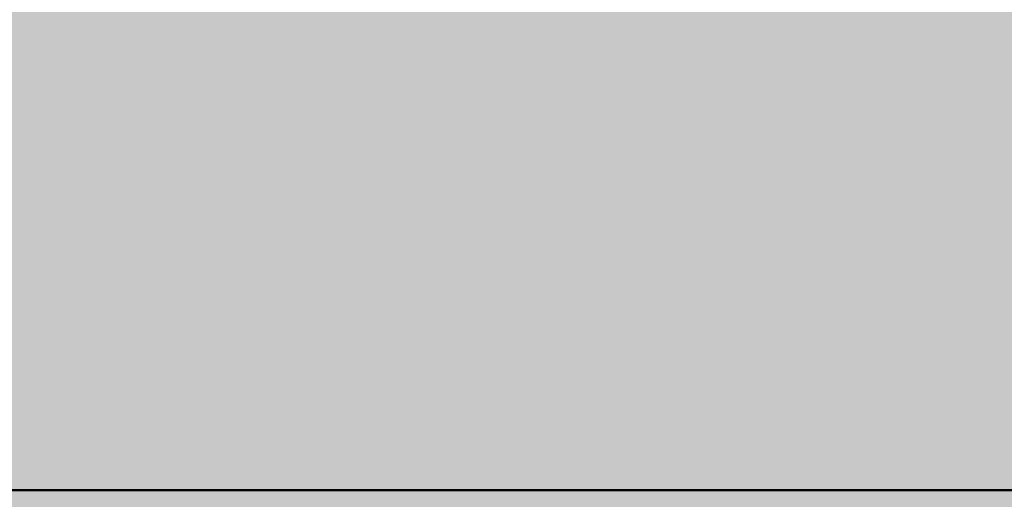
# Model space of a CAD drawing. Units: millimetres. Extents: x 0 to 2267, y 0 to 1823.
# Tile 145 of 256: x 1823.16 to 1833.61, y 1117.32 to 1122.41. Entities that reach past the tile are written whole.
import ezdxf

# ---------------------------------------------------------------- set-up
doc = ezdxf.new("R2010")
doc.units = ezdxf.units.MM
doc.header["$MEASUREMENT"] = 0
for name, color, linetype, lineweight in [('M-DIMS', 2, 'Continuous', 25), ('M-HATC', 252, 'Continuous', 18), ('M-OUTL', 7, 'Continuous', 50)]:
    doc.layers.add(name, color=color, linetype=linetype, lineweight=lineweight)
doc.styles.get("Standard").update_dxf_attribs({"font": 'arial.ttf'})
doc.dimstyles.get("Standard").update_dxf_attribs({"dimtxt": 7, "dimasz": 4, "dimexe": 0.18, "dimexo": 0.0625, "dimgap": 0.09, "dimtad": 0, "dimdec": 0, "dimzin": 0, "dimdsep": 46, "dimtxsty": 'Standard', "dimcen": 0.09, "dimadec": 0, "dimazin": 0, "dimtfac": 1, "dimtdec": 0, "dimtofl": 0, "dimtmove": 0, "dimatfit": 3, "dimfxl": 1, "dimtolj": 1, "dimtzin": 0, "dimarcsym": 0})

# ---------------------------------------------------------------- blocks, each defined once
blk = doc.blocks.new('*D1')
at = {"layer": 'Defpoints', "color": 0, "transparency": 16777216}
for p in [(1593.429, 1127.417), (1843.429, 1127.417), (1843.429, 955.628)]:
    blk.add_point(p, dxfattribs=at)
at = {"layer": 'M-DIMS', "color": 0, "lineweight": -2, "transparency": 16777216}
for p, q in [((1593.429, 1127.355), (1593.429, 955.448)), ((1843.429, 1127.355), (1843.429, 955.448)), ((1597.429, 955.628), (1710.558, 955.628)), ((1839.429, 955.628), (1726.3, 955.628))]:
    blk.add_line(p, q, dxfattribs=at)
at = {"layer": 'M-DIMS', "color": 0, "transparency": 16777216}
for points in [[(1597.429, 956.294), (1597.429, 954.961), (1593.429, 955.628)], [(1839.429, 956.294), (1839.429, 954.961), (1843.429, 955.628)]]:
    blk.add_solid(points, dxfattribs=at)
at = {"layer": 'M-DIMS', "color": 0, "transparency": 16777216, "insert": (1718.429, 955.628), "char_height": 7, "attachment_point": 5}
blk.add_mtext('\\A1;250', dxfattribs=at)

msp = doc.modelspace()

# ---------------------------------------------------------------- hatches: boundary and pattern name
at = {"layer": 'M-HATC'}
h = msp.add_hatch(color=256, dxfattribs=at)
h.dxf.hatch_style = 1
h.paths.add_polyline_path([(2065.771, 1618.062, 0.236068), (2055.771, 1638.062), (1381.087, 1638.062, 0.236068), (1371.087, 1618.062), (1371.087, 1603.062), (2055.771, 1603.062), (2065.771, 1603.062)])
h.paths.add_polyline_path([(2062.772, 1550.296), (2062.772, 1560.296), (1374.086, 1560.296), (1374.086, 1550.296), (1374.086, 1540.296), (1384.086, 1540.296), (1389.086, 1540.296), (2062.772, 1540.296)])
h.paths.add_polyline_path([(1930.929, 1282.766), (1505.929, 1282.766), (1587.628, 1235.597, 0.131652), (1600.128, 1232.247), (1836.73, 1232.247, 0.131652), (1849.23, 1235.597)])
h.paths.add_polyline_path([(1930.929, 1117.417), (1905.929, 1117.417), (1505.929, 1117.417), (1505.929, 1077.417), (1930.929, 1077.417)])
h = msp.add_hatch(color=256, dxfattribs=at)
h.dxf.hatch_style = 1
h.paths.add_polyline_path([(2055.771, 1603.062), (1381.087, 1603.062), (1381.087, 1598.062), (2055.771, 1598.062)])
h.paths.add_polyline_path([(2055.771, 1598.062), (1381.087, 1598.062), (1381.087, 1593.062), (2055.771, 1593.062)])
h.paths.add_polyline_path([(2051.307, 1536.761), (1385.55, 1536.761), (1385.55, 1526.761), (1387.55, 1526.761), (1388.537, 1525.053), (1385.332, 1521.233), (1385.332, 1521.223), (2050.254, 1522.749), (2048.321, 1525.053), (2049.307, 1526.761), (2051.307, 1526.761)])
edge = h.paths.add_edge_path()
edge.add_arc((1847.535, 1379.149), 135, 222.60306, 222.89085, ccw=False)
edge.add_line((1748.166, 1287.766), (1683.092, 1287.766))
edge.add_arc((1583.724, 1379.149), 135, 317.10915, 317.39694, ccw=False)
edge.add_arc((1678.969, 1290.671), 5, 222.8909, 317.1091, ccw=False)
edge.add_arc((1774.213, 1379.149), 135, 222.60306, 222.89085, ccw=False)
edge.add_line((1674.845, 1287.766), (1609.771, 1287.766))
edge.add_arc((1510.403, 1379.149), 135, 317.10915, 317.39694, ccw=False)
edge.add_arc((1605.647, 1290.671), 5, 222.8909, 317.1091, ccw=False)
edge.add_arc((1700.892, 1379.149), 135, 222.60306, 222.89085, ccw=False)
edge.add_line((1601.524, 1287.766), (1536.45, 1287.766))
edge.add_arc((1437.081, 1379.149), 135, 317.10915, 317.39694, ccw=False)
edge.add_arc((1532.326, 1290.671), 5, 222.8909, 317.1091, ccw=False)
edge.add_arc((1627.571, 1379.149), 135, 222.60306, 222.89085, ccw=False)
edge.add_line((1528.203, 1287.766), (1505.929, 1287.766))
edge.add_spline(control_points=[(1505.929, 1287.766), (1504.262, 1287.766), (1504.262, 1282.766), (1505.929, 1282.766)], knot_values=[0, 0, 0, 0, 5, 5, 5, 5], degree=3, periodic=0)
edge.add_line((1505.929, 1282.766), (1930.929, 1282.766))
edge.add_spline(control_points=[(1930.929, 1282.766), (1932.596, 1282.766), (1932.596, 1287.766), (1930.929, 1287.766)], knot_values=[0, 0, 0, 0, 5, 5, 5, 5], degree=3, periodic=0)
edge.add_line((1930.929, 1287.766), (1903.056, 1287.766))
edge.add_arc((1803.688, 1379.149), 135, 317.10915, 317.39694, ccw=False)
edge.add_arc((1898.932, 1290.671), 5, 222.8909, 317.1091, ccw=False)
edge.add_arc((1994.177, 1379.149), 135, 222.60306, 222.89085, ccw=False)
edge.add_line((1894.809, 1287.766), (1829.735, 1287.766))
edge.add_arc((1730.366, 1379.149), 135, 317.10915, 317.39694, ccw=False)
edge.add_arc((1825.611, 1290.671), 5, 222.8909, 317.1091, ccw=False)
edge.add_arc((1920.856, 1379.149), 135, 222.60306, 222.89085, ccw=False)
edge.add_line((1821.487, 1287.766), (1756.413, 1287.766))
edge.add_arc((1657.045, 1379.149), 135, 317.10915, 317.39694, ccw=False)
edge.add_arc((1752.29, 1290.671), 5, 222.8909, 317.1091, ccw=False)
edge = h.paths.add_edge_path()
edge.add_spline(control_points=[(1843.429, 1227.247), (1845.096, 1227.247), (1845.096, 1232.247), (1843.429, 1232.247)], knot_values=[0, 0, 0, 0, 5, 5, 5, 5], degree=3, periodic=0)
edge.add_line((1843.429, 1232.247), (1593.429, 1232.247))
edge.add_spline(control_points=[(1593.429, 1232.247), (1591.762, 1232.247), (1591.762, 1227.247), (1593.429, 1227.247)], knot_values=[0, 0, 0, 0, 5, 5, 5, 5], degree=3, periodic=0)
edge.add_line((1593.429, 1227.247), (1843.429, 1227.247))
h.paths.add_polyline_path([(1905.929, 1127.417), (1530.929, 1127.417, 0.414214), (1520.929, 1117.417), (1530.929, 1117.417), (1915.929, 1117.417, 0.414214)])
edge = h.paths.add_edge_path()
edge.add_arc((1397.086, 1498.408), 12.73, 90.7821, 190.8787, ccw=False)
edge.add_line((1396.912, 1511.136), (1428.01, 1511.349))
edge.add_line((1428.01, 1511.349), (1433.01, 1511.349))
edge.add_line((1433.01, 1511.349), (1434.439, 1511.349))
edge.add_arc((1419.474, 1498.08), 20, 41.561, 74.0821)
edge.add_line((1424.959, 1517.314), (1399.935, 1517.256))
edge.add_spline(control_points=[(1399.931, 1517.256), (1399.884, 1517.213), (1399.833, 1517.169), (1399.777, 1517.124)], knot_values=[11.567499, 11.567499, 11.567499, 11.567499, 11.814249, 11.814249, 11.814249, 11.814249], degree=3, periodic=0)
edge.add_spline(control_points=[(1399.633, 1517.01), (1399.583, 1516.972), (1399.531, 1516.934), (1399.476, 1516.895)], knot_values=[11.167718, 11.167718, 11.167718, 11.167718, 11.365188, 11.365188, 11.365188, 11.365188], degree=3, periodic=0)
edge.add_spline(control_points=[(1399.34, 1516.8), (1399.151, 1516.672), (1398.938, 1516.538), (1398.704, 1516.399)], knot_values=[10.376405, 10.376405, 10.376405, 10.376405, 11.00994, 11.00994, 11.00994, 11.00994], degree=3, periodic=0)
edge.add_spline(control_points=[(1398.657, 1516.372), (1398.579, 1516.326), (1398.498, 1516.28), (1398.415, 1516.233)], knot_values=[10.125175, 10.125175, 10.125175, 10.125175, 10.334406, 10.334406, 10.334406, 10.334406], degree=3, periodic=0)
edge.add_spline(control_points=[(1398.264, 1516.149), (1398.196, 1516.111), (1398.126, 1516.073), (1398.055, 1516.035)], knot_values=[9.832246, 9.832246, 9.832246, 9.832246, 9.999658, 9.999658, 9.999658, 9.999658], degree=3, periodic=0)
edge.add_spline(control_points=[(1397.999, 1516.005), (1397.731, 1515.862), (1397.446, 1515.717), (1397.147, 1515.571)], knot_values=[9.161808, 9.161808, 9.161808, 9.161808, 9.787769, 9.787769, 9.787769, 9.787769], degree=3, periodic=0)
edge.add_spline(control_points=[(1397.147, 1515.571), (1396.842, 1515.423), (1396.522, 1515.274), (1396.191, 1515.126)], knot_values=[8.524455, 8.524455, 8.524455, 8.524455, 9.161808, 9.161808, 9.161808, 9.161808], degree=3, periodic=0)
edge.add_spline(control_points=[(1396.078, 1515.076), (1395.985, 1515.035), (1395.892, 1514.994), (1395.798, 1514.953)], knot_values=[8.275193, 8.275193, 8.275193, 8.275193, 8.451726, 8.451726, 8.451726, 8.451726], degree=3, periodic=0)
edge.add_spline(control_points=[(1395.602, 1514.869), (1395.5, 1514.826), (1395.397, 1514.782), (1395.293, 1514.739)], knot_values=[7.962917, 7.962917, 7.962917, 7.962917, 8.152764, 8.152764, 8.152764, 8.152764], degree=3, periodic=0)
edge.add_spline(control_points=[(1395.212, 1514.706), (1394.828, 1514.547), (1394.435, 1514.393), (1394.036, 1514.244)], knot_values=[7.21254, 7.21254, 7.21254, 7.21254, 7.913148, 7.913148, 7.913148, 7.913148], degree=3, periodic=0)
edge.add_spline(control_points=[(1394.036, 1514.244), (1393.708, 1514.121), (1393.375, 1514.003), (1393.043, 1513.889)], knot_values=[6.633733, 6.633733, 6.633733, 6.633733, 7.21254, 7.21254, 7.21254, 7.21254], degree=3, periodic=0)
edge.add_spline(control_points=[(1392.821, 1513.815), (1392.72, 1513.781), (1392.618, 1513.748), (1392.517, 1513.715)], knot_values=[6.328796, 6.328796, 6.328796, 6.328796, 6.505493, 6.505493, 6.505493, 6.505493], degree=3, periodic=0)
edge.add_spline(control_points=[(1392.517, 1513.715), (1392.319, 1513.652), (1392.121, 1513.59), (1391.924, 1513.531)], knot_values=[5.984605, 5.984605, 5.984605, 5.984605, 6.328796, 6.328796, 6.328796, 6.328796], degree=3, periodic=0)
edge.add_spline(control_points=[(1391.792, 1513.491), (1391.312, 1513.35), (1390.838, 1513.224), (1390.378, 1513.117)], knot_values=[5.066697, 5.066697, 5.066697, 5.066697, 5.907055, 5.907055, 5.907055, 5.907055], degree=3, periodic=0)
edge.add_spline(control_points=[(1390.378, 1513.117), (1390.18, 1513.071), (1389.984, 1513.028), (1389.791, 1512.99)], knot_values=[4.70367, 4.70367, 4.70367, 4.70367, 5.066695, 5.066695, 5.066695, 5.066695], degree=3, periodic=0)
edge.add_spline(control_points=[(1389.422, 1512.92), (1389.246, 1512.889), (1389.073, 1512.862), (1388.904, 1512.838)], knot_values=[4.130571, 4.130571, 4.130571, 4.130571, 4.469816, 4.469816, 4.469816, 4.469816], degree=3, periodic=0)
edge.add_spline(control_points=[(1388.904, 1512.838), (1388.591, 1512.795), (1388.291, 1512.764), (1388.007, 1512.749)], knot_values=[3.504031, 3.504031, 3.504031, 3.504031, 4.130571, 4.130571, 4.130571, 4.130571], degree=3, periodic=0)
edge.add_spline(control_points=[(1387.936, 1512.746), (1387.854, 1512.742), (1387.773, 1512.74), (1387.694, 1512.739)], knot_values=[3.268866, 3.268866, 3.268866, 3.268866, 3.451164, 3.451164, 3.451164, 3.451164], degree=3, periodic=0)
edge.add_spline(control_points=[(1387.335, 1512.744), (1387.208, 1512.75), (1387.085, 1512.76), (1386.967, 1512.774)], knot_values=[2.670686, 2.670686, 2.670686, 2.670686, 2.984, 2.984, 2.984, 2.984], degree=3, periodic=0)
edge.add_spline(control_points=[(1386.833, 1512.792), (1386.821, 1512.794), (1386.809, 1512.796), (1386.797, 1512.798)], knot_values=[2.516981, 2.516981, 2.516981, 2.516981, 2.549528, 2.549528, 2.549528, 2.549528], degree=3, periodic=0)
edge.add_spline(control_points=[(1386.453, 1512.873), (1386.426, 1512.881), (1386.399, 1512.889), (1386.373, 1512.897)], knot_values=[2.095869, 2.095869, 2.095869, 2.095869, 2.17941, 2.17941, 2.17941, 2.17941], degree=3, periodic=0)
edge.add_spline(control_points=[(1386.069, 1513.019), (1386.063, 1513.022), (1386.058, 1513.025), (1386.052, 1513.028)], knot_values=[1.72453, 1.72453, 1.72453, 1.72453, 1.745933, 1.745933, 1.745933, 1.745933], degree=3, periodic=0)
edge.add_arc((1399.474, 1498.08), 20, 131.8243, 180)
edge.add_arc((1630.334, 1505.548), 250.971, 181.70518, 236.42798)
edge.add_arc((1605.34, 1483.304), 218.782, 238.66083, 243.34961)
edge.add_arc((1647.091, 1510.359), 262.899, 183.12984, 237.85344, ccw=False)
h.paths.add_polyline_path([(1406.537, 1391.964, 0.149382), (1491.551, 1296.442, -0.129517)], flags=17)
edge = h.paths.add_edge_path()
edge.add_arc((2037.384, 1498.08), 20, 0, 48.2659)
edge.add_spline(control_points=[(2050.697, 1513.005), (2050.651, 1512.985), (2050.603, 1512.966), (2050.554, 1512.948)], knot_values=[1.835652, 1.835652, 1.835652, 1.835652, 2.000781, 2.000781, 2.000781, 2.000781], degree=3, periodic=0)
edge.add_spline(control_points=[(2050.462, 1512.917), (2050.479, 1512.922), (2050.496, 1512.928), (2050.513, 1512.934)], knot_values=[2.045477, 2.045477, 2.045477, 2.045477, 2.101389, 2.101389, 2.101389, 2.101389], degree=3, periodic=0)
edge.add_spline(control_points=[(2050.129, 1512.834), (2050.198, 1512.847), (2050.266, 1512.862), (2050.331, 1512.879)], knot_values=[2.237629, 2.237629, 2.237629, 2.237629, 2.435841, 2.435841, 2.435841, 2.435841], degree=3, periodic=0)
edge.add_spline(control_points=[(2050.095, 1512.828), (2050.106, 1512.83), (2050.118, 1512.832), (2050.129, 1512.834)], knot_values=[2.435841, 2.435841, 2.435841, 2.435841, 2.468321, 2.468321, 2.468321, 2.468321], degree=3, periodic=0)
edge.add_spline(control_points=[(2049.784, 1512.785), (2049.855, 1512.792), (2049.924, 1512.801), (2049.992, 1512.811)], knot_values=[2.563852, 2.563852, 2.563852, 2.563852, 2.748541, 2.748541, 2.748541, 2.748541], degree=3, periodic=0)
edge.add_spline(control_points=[(2049.405, 1512.762), (2049.536, 1512.765), (2049.663, 1512.773), (2049.784, 1512.785)], knot_values=[2.748541, 2.748541, 2.748541, 2.748541, 3.064882, 3.064882, 3.064882, 3.064882], degree=3, periodic=0)
edge.add_spline(control_points=[(2049.17, 1512.76), (2049.234, 1512.759), (2049.297, 1512.759), (2049.358, 1512.761)], knot_values=[3.102309, 3.102309, 3.102309, 3.102309, 3.2503, 3.2503, 3.2503, 3.2503], degree=3, periodic=0)
edge.add_spline(control_points=[(2048.857, 1512.769), (2048.964, 1512.764), (2049.068, 1512.761), (2049.17, 1512.76)], knot_values=[3.2503, 3.2503, 3.2503, 3.2503, 3.486069, 3.486069, 3.486069, 3.486069], degree=3, periodic=0)
edge.add_spline(control_points=[(2048.692, 1512.779), (2048.373, 1512.801), (2048.035, 1512.841), (2047.682, 1512.897)], knot_values=[3.606429, 3.606429, 3.606429, 3.606429, 4.2989, 4.2989, 4.2989, 4.2989], degree=3, periodic=0)
edge.add_spline(control_points=[(2047.682, 1512.897), (2047.546, 1512.919), (2047.408, 1512.942), (2047.268, 1512.969)], knot_values=[4.2989, 4.2989, 4.2989, 4.2989, 4.565769, 4.565769, 4.565769, 4.565769], degree=3, periodic=0)
edge.add_spline(control_points=[(2047.268, 1512.969), (2047.145, 1512.991), (2047.021, 1513.016), (2046.895, 1513.042)], knot_values=[4.565769, 4.565769, 4.565769, 4.565769, 4.799971, 4.799971, 4.799971, 4.799971], degree=3, periodic=0)
edge.add_spline(control_points=[(2046.895, 1513.042), (2046.529, 1513.119), (2046.151, 1513.209), (2045.768, 1513.311)], knot_values=[4.799971, 4.799971, 4.799971, 4.799971, 5.483718, 5.483718, 5.483718, 5.483718], degree=3, periodic=0)
edge.add_spline(control_points=[(2045.768, 1513.311), (2045.372, 1513.415), (2044.97, 1513.532), (2044.566, 1513.659)], knot_values=[5.483718, 5.483718, 5.483718, 5.483718, 6.187866, 6.187866, 6.187866, 6.187866], degree=3, periodic=0)
edge.add_spline(control_points=[(2044.566, 1513.659), (2044.415, 1513.706), (2044.263, 1513.755), (2044.112, 1513.805)], knot_values=[6.187866, 6.187866, 6.187866, 6.187866, 6.451551, 6.451551, 6.451551, 6.451551], degree=3, periodic=0)
edge.add_spline(control_points=[(2044.112, 1513.805), (2043.997, 1513.843), (2043.882, 1513.881), (2043.767, 1513.92)], knot_values=[6.451551, 6.451551, 6.451551, 6.451551, 6.651434, 6.651434, 6.651434, 6.651434], degree=3, periodic=0)
edge.add_spline(control_points=[(2043.767, 1513.92), (2043.372, 1514.055), (2042.977, 1514.198), (2042.589, 1514.346)], knot_values=[6.651434, 6.651434, 6.651434, 6.651434, 7.338879, 7.338879, 7.338879, 7.338879], degree=3, periodic=0)
edge.add_spline(control_points=[(2042.589, 1514.346), (2042.164, 1514.507), (2041.746, 1514.675), (2041.341, 1514.846)], knot_values=[7.338879, 7.338879, 7.338879, 7.338879, 8.089209, 8.089209, 8.089209, 8.089209], degree=3, periodic=0)
edge.add_spline(control_points=[(2041.341, 1514.846), (2041.103, 1514.946), (2040.869, 1515.048), (2040.64, 1515.15)], knot_values=[8.089209, 8.089209, 8.089209, 8.089209, 8.529587, 8.529587, 8.529587, 8.529587], degree=3, periodic=0)
edge.add_spline(control_points=[(2040.51, 1515.209), (2040.082, 1515.402), (2039.675, 1515.597), (2039.295, 1515.789)], knot_values=[8.613818, 8.613818, 8.613818, 8.613818, 9.44571, 9.44571, 9.44571, 9.44571], degree=3, periodic=0)
edge.add_spline(control_points=[(2039.295, 1515.789), (2039.062, 1515.907), (2038.839, 1516.025), (2038.629, 1516.14)], knot_values=[9.44571, 9.44571, 9.44571, 9.44571, 9.956404, 9.956404, 9.956404, 9.956404], degree=3, periodic=0)
edge.add_spline(control_points=[(2038.629, 1516.14), (2038.519, 1516.2), (2038.412, 1516.26), (2038.309, 1516.319)], knot_values=[9.956404, 9.956404, 9.956404, 9.956404, 10.223542, 10.223542, 10.223542, 10.223542], degree=3, periodic=0)
edge.add_spline(control_points=[(2038.309, 1516.319), (2038.214, 1516.374), (2038.122, 1516.428), (2038.033, 1516.481)], knot_values=[10.223542, 10.223542, 10.223542, 10.223542, 10.47051, 10.47051, 10.47051, 10.47051], degree=3, periodic=0)
edge.add_spline(control_points=[(2038.033, 1516.481), (2037.786, 1516.63), (2037.564, 1516.773), (2037.372, 1516.909)], knot_values=[10.47051, 10.47051, 10.47051, 10.47051, 11.15767, 11.15767, 11.15767, 11.15767], degree=3, periodic=0)
edge.add_spline(control_points=[(2037.372, 1516.909), (2037.279, 1516.975), (2037.193, 1517.04), (2037.114, 1517.102)], knot_values=[11.15767, 11.15767, 11.15767, 11.15767, 11.49227, 11.49227, 11.49227, 11.49227], degree=3, periodic=0)
edge.add_spline(control_points=[(2036.856, 1517.326), (2036.915, 1517.269), (2036.981, 1517.21), (2037.056, 1517.149)], knot_values=[11.577341, 11.577341, 11.577341, 11.577341, 11.91035, 11.91035, 11.91035, 11.91035], degree=3, periodic=0)
edge.add_spline(control_points=[(2036.807, 1517.375), (2036.823, 1517.359), (2036.839, 1517.342), (2036.856, 1517.326)], knot_values=[11.91035, 11.91035, 11.91035, 11.91035, 12.007402, 12.007402, 12.007402, 12.007402], degree=3, periodic=0)
edge.add_spline(control_points=[(2036.702, 1517.494), (2036.71, 1517.483), (2036.72, 1517.472), (2036.729, 1517.461)], knot_values=[12.184155, 12.184155, 12.184155, 12.184155, 12.255409, 12.255409, 12.255409, 12.255409], degree=3, periodic=0)
edge.add_spline(control_points=[(2036.616, 1517.621), (2036.62, 1517.613), (2036.624, 1517.606), (2036.629, 1517.598)], knot_values=[12.487913, 12.487913, 12.487913, 12.487913, 12.541035, 12.541035, 12.541035, 12.541035], degree=3, periodic=0)
edge.add_spline(control_points=[(2036.563, 1517.786), (2036.564, 1517.779), (2036.564, 1517.773), (2036.565, 1517.766)], knot_values=[12.911761, 12.911761, 12.911761, 12.911761, 12.968286, 12.968286, 12.968286, 12.968286], degree=3, periodic=0)
edge.add_spline(control_points=[(2036.617, 1517.93), (2036.612, 1517.926), (2036.609, 1517.921), (2036.605, 1517.916)], knot_values=[13.382527, 13.382527, 13.382527, 13.382527, 13.433791, 13.433791, 13.433791, 13.433791], degree=3, periodic=0)
edge.add_spline(control_points=[(2036.749, 1518.017), (2036.736, 1518.012), (2036.724, 1518.006), (2036.712, 1518)], knot_values=[13.726299, 13.726299, 13.726299, 13.726299, 13.809928, 13.809928, 13.809928, 13.809928], degree=3, periodic=0)
edge.add_spline(control_points=[(2036.86, 1518.053), (2036.839, 1518.047), (2036.818, 1518.042), (2036.799, 1518.035)], knot_values=[13.910887, 13.910887, 13.910887, 13.910887, 14.02153, 14.02153, 14.02153, 14.02153], degree=3, periodic=0)
edge.add_line((2036.964, 1518.08), (2032.384, 1518.08))
edge.add_line((2032.384, 1518.08), (2027.384, 1518.08))
edge.add_line((2027.384, 1518.08), (2022.384, 1518.08))
edge.add_line((2022.384, 1518.08), (2017.384, 1518.08))
edge.add_arc((2017.384, 1498.08), 20, 90, 138.439)
edge.add_line((2002.419, 1511.349), (2003.848, 1511.349))
edge.add_line((2003.848, 1511.349), (2008.848, 1511.349))
edge.add_line((2008.848, 1511.349), (2039.772, 1511.138))
edge.add_arc((2039.772, 1498.408), 12.73, -10.8787, 90, ccw=False)
edge.add_arc((1789.767, 1510.359), 262.899, 302.14656, 356.87016, ccw=False)
edge.add_arc((1831.518, 1483.304), 218.782, 296.65039, 301.33917)
edge.add_arc((1806.524, 1505.548), 250.971, 303.57202, 358.29482)
h.paths.add_polyline_path([(2030.321, 1391.964, -0.129517), (1945.307, 1296.442, 0.149382)], flags=17)
edge = h.paths.add_edge_path()
edge.add_spline(control_points=[(2037.246, 1518.082), (2037.29, 1518.081), (2037.336, 1518.08), (2037.384, 1518.08)], knot_values=[0.000012, 0.000012, 0.000012, 0.000012, 0.144754, 0.144754, 0.144754, 0.144754], degree=3, periodic=0)
edge.add_line((2037.336, 1518.08), (2037.01, 1518.08))
edge.add_spline(control_points=[(2037.01, 1518.08), (2036.982, 1518.077), (2036.956, 1518.073), (2036.931, 1518.068)], knot_values=[14.13465, 14.13465, 14.13465, 14.13465, 14.247197, 14.247197, 14.247197, 14.247197], degree=3, periodic=0)
edge.add_spline(control_points=[(2036.931, 1518.068), (2036.928, 1518.067), (2036.924, 1518.067), (2036.921, 1518.066)], knot_values=[14.118315, 14.118315, 14.118315, 14.118315, 14.13465, 14.13465, 14.13465, 14.13465], degree=3, periodic=0)
edge.add_spline(control_points=[(2036.921, 1518.066), (2036.912, 1518.064), (2036.903, 1518.063), (2036.895, 1518.061)], knot_values=[14.078086, 14.078086, 14.078086, 14.078086, 14.118315, 14.118315, 14.118315, 14.118315], degree=3, periodic=0)
edge.add_spline(control_points=[(2036.895, 1518.061), (2036.883, 1518.058), (2036.872, 1518.056), (2036.86, 1518.053)], knot_values=[14.02153, 14.02153, 14.02153, 14.02153, 14.078086, 14.078086, 14.078086, 14.078086], degree=3, periodic=0)
edge.add_spline(control_points=[(2036.86, 1518.053), (2036.839, 1518.047), (2036.818, 1518.042), (2036.799, 1518.035)], knot_values=[13.910887, 13.910887, 13.910887, 13.910887, 14.02153, 14.02153, 14.02153, 14.02153], degree=3, periodic=0)
edge.add_spline(control_points=[(2036.799, 1518.035), (2036.798, 1518.035), (2036.797, 1518.035), (2036.797, 1518.035)], knot_values=[13.906906, 13.906906, 13.906906, 13.906906, 13.910887, 13.910887, 13.910887, 13.910887], degree=3, periodic=0)
edge.add_spline(control_points=[(2036.797, 1518.035), (2036.788, 1518.032), (2036.78, 1518.029), (2036.772, 1518.026)], knot_values=[13.857826, 13.857826, 13.857826, 13.857826, 13.906906, 13.906906, 13.906906, 13.906906], degree=3, periodic=0)
edge.add_spline(control_points=[(2036.772, 1518.026), (2036.764, 1518.023), (2036.756, 1518.02), (2036.749, 1518.017)], knot_values=[13.809928, 13.809928, 13.809928, 13.809928, 13.857826, 13.857826, 13.857826, 13.857826], degree=3, periodic=0)
edge.add_spline(control_points=[(2036.749, 1518.017), (2036.736, 1518.012), (2036.724, 1518.006), (2036.712, 1518)], knot_values=[13.726299, 13.726299, 13.726299, 13.726299, 13.809928, 13.809928, 13.809928, 13.809928], degree=3, periodic=0)
edge.add_spline(control_points=[(2036.712, 1518), (2036.712, 1518), (2036.712, 1518), (2036.711, 1518)], knot_values=[13.723993, 13.723993, 13.723993, 13.723993, 13.726299, 13.726299, 13.726299, 13.726299], degree=3, periodic=0)
edge.add_spline(control_points=[(2036.711, 1518), (2036.706, 1517.997), (2036.701, 1517.994), (2036.696, 1517.992)], knot_values=[13.686536, 13.686536, 13.686536, 13.686536, 13.723993, 13.723993, 13.723993, 13.723993], degree=3, periodic=0)
edge.add_spline(control_points=[(2036.696, 1517.992), (2036.692, 1517.989), (2036.687, 1517.987), (2036.683, 1517.984)], knot_values=[13.651251, 13.651251, 13.651251, 13.651251, 13.686536, 13.686536, 13.686536, 13.686536], degree=3, periodic=0)
edge.add_spline(control_points=[(2036.683, 1517.984), (2036.676, 1517.98), (2036.67, 1517.976), (2036.664, 1517.971)], knot_values=[13.596804, 13.596804, 13.596804, 13.596804, 13.651251, 13.651251, 13.651251, 13.651251], degree=3, periodic=0)
edge.add_spline(control_points=[(2036.664, 1517.971), (2036.664, 1517.971), (2036.663, 1517.971), (2036.663, 1517.971)], knot_values=[13.593956, 13.593956, 13.593956, 13.593956, 13.596804, 13.596804, 13.596804, 13.596804], degree=3, periodic=0)
edge.add_spline(control_points=[(2036.663, 1517.971), (2036.66, 1517.969), (2036.658, 1517.967), (2036.655, 1517.965)], knot_values=[13.570322, 13.570322, 13.570322, 13.570322, 13.593956, 13.593956, 13.593956, 13.593956], degree=3, periodic=0)
edge.add_spline(control_points=[(2036.655, 1517.965), (2036.653, 1517.963), (2036.65, 1517.961), (2036.647, 1517.959)], knot_values=[13.545477, 13.545477, 13.545477, 13.545477, 13.570322, 13.570322, 13.570322, 13.570322], degree=3, periodic=0)
edge.add_spline(control_points=[(2036.647, 1517.959), (2036.647, 1517.959), (2036.647, 1517.959), (2036.647, 1517.959)], knot_values=[13.543931, 13.543931, 13.543931, 13.543931, 13.545477, 13.545477, 13.545477, 13.545477], degree=3, periodic=0)
edge.add_spline(control_points=[(2036.647, 1517.959), (2036.641, 1517.954), (2036.636, 1517.949), (2036.631, 1517.945)], knot_values=[13.488237, 13.488237, 13.488237, 13.488237, 13.543931, 13.543931, 13.543931, 13.543931], degree=3, periodic=0)
edge.add_spline(control_points=[(2036.631, 1517.945), (2036.628, 1517.942), (2036.626, 1517.94), (2036.623, 1517.937)], knot_values=[13.460307, 13.460307, 13.460307, 13.460307, 13.488237, 13.488237, 13.488237, 13.488237], degree=3, periodic=0)
edge.add_spline(control_points=[(2036.623, 1517.937), (2036.622, 1517.936), (2036.62, 1517.934), (2036.618, 1517.932)], knot_values=[13.439712, 13.439712, 13.439712, 13.439712, 13.460307, 13.460307, 13.460307, 13.460307], degree=3, periodic=0)
edge.add_spline(control_points=[(2036.618, 1517.932), (2036.618, 1517.931), (2036.617, 1517.931), (2036.617, 1517.93)], knot_values=[13.433791, 13.433791, 13.433791, 13.433791, 13.439712, 13.439712, 13.439712, 13.439712], degree=3, periodic=0)
edge.add_spline(control_points=[(2036.617, 1517.93), (2036.612, 1517.926), (2036.609, 1517.921), (2036.605, 1517.916)], knot_values=[13.382527, 13.382527, 13.382527, 13.382527, 13.433791, 13.433791, 13.433791, 13.433791], degree=3, periodic=0)
edge.add_spline(control_points=[(2036.605, 1517.916), (2036.603, 1517.913), (2036.6, 1517.91), (2036.598, 1517.907)], knot_values=[13.350017, 13.350017, 13.350017, 13.350017, 13.382527, 13.382527, 13.382527, 13.382527], degree=3, periodic=0)
edge.add_spline(control_points=[(2036.598, 1517.907), (2036.597, 1517.906), (2036.596, 1517.904), (2036.595, 1517.903)], knot_values=[13.333922, 13.333922, 13.333922, 13.333922, 13.350017, 13.350017, 13.350017, 13.350017], degree=3, periodic=0)
edge.add_spline(control_points=[(2036.595, 1517.903), (2036.595, 1517.902), (2036.594, 1517.901), (2036.593, 1517.9)], knot_values=[13.323828, 13.323828, 13.323828, 13.323828, 13.333922, 13.333922, 13.333922, 13.333922], degree=3, periodic=0)
edge.add_spline(control_points=[(2036.593, 1517.9), (2036.59, 1517.895), (2036.588, 1517.891), (2036.585, 1517.886)], knot_values=[13.277545, 13.277545, 13.277545, 13.277545, 13.323828, 13.323828, 13.323828, 13.323828], degree=3, periodic=0)
edge.add_spline(control_points=[(2036.585, 1517.886), (2036.584, 1517.883), (2036.582, 1517.879), (2036.58, 1517.875)], knot_values=[13.240119, 13.240119, 13.240119, 13.240119, 13.277545, 13.277545, 13.277545, 13.277545], degree=3, periodic=0)
edge.add_spline(control_points=[(2036.58, 1517.875), (2036.58, 1517.874), (2036.579, 1517.873), (2036.578, 1517.872)], knot_values=[13.228211, 13.228211, 13.228211, 13.228211, 13.240119, 13.240119, 13.240119, 13.240119], degree=3, periodic=0)
edge.add_spline(control_points=[(2036.578, 1517.872), (2036.578, 1517.87), (2036.577, 1517.869), (2036.577, 1517.868)], knot_values=[13.215717, 13.215717, 13.215717, 13.215717, 13.228211, 13.228211, 13.228211, 13.228211], degree=3, periodic=0)
edge.add_spline(control_points=[(2036.577, 1517.868), (2036.575, 1517.864), (2036.574, 1517.86), (2036.573, 1517.857)], knot_values=[13.179847, 13.179847, 13.179847, 13.179847, 13.215717, 13.215717, 13.215717, 13.215717], degree=3, periodic=0)
edge.add_spline(control_points=[(2036.573, 1517.857), (2036.571, 1517.851), (2036.57, 1517.846), (2036.569, 1517.841)], knot_values=[13.132017, 13.132017, 13.132017, 13.132017, 13.179847, 13.179847, 13.179847, 13.179847], degree=3, periodic=0)
edge.add_spline(control_points=[(2036.569, 1517.841), (2036.568, 1517.84), (2036.568, 1517.839), (2036.568, 1517.838)], knot_values=[13.122482, 13.122482, 13.122482, 13.122482, 13.132017, 13.132017, 13.132017, 13.132017], degree=3, periodic=0)
edge.add_spline(control_points=[(2036.568, 1517.838), (2036.568, 1517.836), (2036.567, 1517.835), (2036.567, 1517.833)], knot_values=[13.105592, 13.105592, 13.105592, 13.105592, 13.122482, 13.122482, 13.122482, 13.122482], degree=3, periodic=0)
edge.add_spline(control_points=[(2036.567, 1517.833), (2036.566, 1517.829), (2036.566, 1517.826), (2036.565, 1517.822)], knot_values=[13.074063, 13.074063, 13.074063, 13.074063, 13.105592, 13.105592, 13.105592, 13.105592], degree=3, periodic=0)
edge.add_spline(control_points=[(2036.565, 1517.822), (2036.565, 1517.822), (2036.565, 1517.822), (2036.565, 1517.822)], knot_values=[13.074043, 13.074043, 13.074043, 13.074043, 13.074063, 13.074063, 13.074063, 13.074063], degree=3, periodic=0)
edge.add_spline(control_points=[(2036.565, 1517.822), (2036.564, 1517.816), (2036.564, 1517.811), (2036.564, 1517.805)], knot_values=[13.021884, 13.021884, 13.021884, 13.021884, 13.074043, 13.074043, 13.074043, 13.074043], degree=3, periodic=0)
edge.add_spline(control_points=[(2036.564, 1517.805), (2036.564, 1517.804), (2036.564, 1517.803), (2036.564, 1517.803)], knot_values=[13.01674, 13.01674, 13.01674, 13.01674, 13.021884, 13.021884, 13.021884, 13.021884], degree=3, periodic=0)
edge.add_spline(control_points=[(2036.564, 1517.803), (2036.563, 1517.801), (2036.563, 1517.798), (2036.563, 1517.796)], knot_values=[12.996438, 12.996438, 12.996438, 12.996438, 13.01674, 13.01674, 13.01674, 13.01674], degree=3, periodic=0)
edge.add_spline(control_points=[(2036.563, 1517.796), (2036.563, 1517.793), (2036.563, 1517.789), (2036.563, 1517.786)], knot_values=[12.968286, 12.968286, 12.968286, 12.968286, 12.996438, 12.996438, 12.996438, 12.996438], degree=3, periodic=0)
edge.add_spline(control_points=[(2036.563, 1517.786), (2036.564, 1517.779), (2036.564, 1517.773), (2036.565, 1517.766)], knot_values=[12.911761, 12.911761, 12.911761, 12.911761, 12.968286, 12.968286, 12.968286, 12.968286], degree=3, periodic=0)
edge.add_spline(control_points=[(2036.565, 1517.766), (2036.565, 1517.766), (2036.565, 1517.766), (2036.565, 1517.766)], knot_values=[12.911017, 12.911017, 12.911017, 12.911017, 12.911761, 12.911761, 12.911761, 12.911761], degree=3, periodic=0)
edge.add_spline(control_points=[(2036.565, 1517.766), (2036.565, 1517.762), (2036.566, 1517.759), (2036.566, 1517.756)], knot_values=[12.88528, 12.88528, 12.88528, 12.88528, 12.911017, 12.911017, 12.911017, 12.911017], degree=3, periodic=0)
edge.add_spline(control_points=[(2036.566, 1517.756), (2036.567, 1517.753), (2036.567, 1517.751), (2036.568, 1517.748)], knot_values=[12.862519, 12.862519, 12.862519, 12.862519, 12.88528, 12.88528, 12.88528, 12.88528], degree=3, periodic=0)
edge.add_spline(control_points=[(2036.568, 1517.748), (2036.568, 1517.747), (2036.568, 1517.747), (2036.568, 1517.746)], knot_values=[12.858885, 12.858885, 12.858885, 12.858885, 12.862519, 12.862519, 12.862519, 12.862519], degree=3, periodic=0)
edge.add_spline(control_points=[(2036.568, 1517.746), (2036.569, 1517.74), (2036.571, 1517.733), (2036.572, 1517.726)], knot_values=[12.8053, 12.8053, 12.8053, 12.8053, 12.858885, 12.858885, 12.858885, 12.858885], degree=3, periodic=0)
edge.add_spline(control_points=[(2036.572, 1517.726), (2036.573, 1517.723), (2036.574, 1517.719), (2036.576, 1517.715)], knot_values=[12.775176, 12.775176, 12.775176, 12.775176, 12.8053, 12.8053, 12.8053, 12.8053], degree=3, periodic=0)
edge.add_spline(control_points=[(2036.576, 1517.715), (2036.576, 1517.713), (2036.577, 1517.71), (2036.578, 1517.708)], knot_values=[12.756759, 12.756759, 12.756759, 12.756759, 12.775176, 12.775176, 12.775176, 12.775176], degree=3, periodic=0)
edge.add_spline(control_points=[(2036.578, 1517.708), (2036.578, 1517.707), (2036.578, 1517.706), (2036.579, 1517.705)], knot_values=[12.748742, 12.748742, 12.748742, 12.748742, 12.756759, 12.756759, 12.756759, 12.756759], degree=3, periodic=0)
edge.add_spline(control_points=[(2036.579, 1517.705), (2036.581, 1517.698), (2036.583, 1517.692), (2036.586, 1517.685)], knot_values=[12.69959, 12.69959, 12.69959, 12.69959, 12.748742, 12.748742, 12.748742, 12.748742], degree=3, periodic=0)
edge.add_spline(control_points=[(2036.586, 1517.685), (2036.588, 1517.68), (2036.59, 1517.675), (2036.592, 1517.669)], knot_values=[12.659038, 12.659038, 12.659038, 12.659038, 12.69959, 12.69959, 12.69959, 12.69959], degree=3, periodic=0)
edge.add_spline(control_points=[(2036.592, 1517.669), (2036.594, 1517.665), (2036.596, 1517.66), (2036.598, 1517.656)], knot_values=[12.626806, 12.626806, 12.626806, 12.626806, 12.659038, 12.659038, 12.659038, 12.659038], degree=3, periodic=0)
edge.add_spline(control_points=[(2036.598, 1517.656), (2036.598, 1517.655), (2036.599, 1517.654), (2036.599, 1517.653)], knot_values=[12.619394, 12.619394, 12.619394, 12.619394, 12.626806, 12.626806, 12.626806, 12.626806], degree=3, periodic=0)
edge.add_spline(control_points=[(2036.599, 1517.653), (2036.604, 1517.642), (2036.61, 1517.632), (2036.616, 1517.621)], knot_values=[12.541039, 12.541039, 12.541039, 12.541039, 12.619394, 12.619394, 12.619394, 12.619394], degree=3, periodic=0)
edge.add_spline(control_points=[(2036.616, 1517.621), (2036.616, 1517.621), (2036.616, 1517.621), (2036.616, 1517.621)], knot_values=[12.541035, 12.541035, 12.541035, 12.541035, 12.541039, 12.541039, 12.541039, 12.541039], degree=3, periodic=0)
edge.add_spline(control_points=[(2036.616, 1517.621), (2036.62, 1517.613), (2036.624, 1517.606), (2036.629, 1517.598)], knot_values=[12.487913, 12.487913, 12.487913, 12.487913, 12.541035, 12.541035, 12.541035, 12.541035], degree=3, periodic=0)
edge.add_spline(control_points=[(2036.629, 1517.598), (2036.633, 1517.592), (2036.637, 1517.585), (2036.641, 1517.579)], knot_values=[12.443982, 12.443982, 12.443982, 12.443982, 12.487913, 12.487913, 12.487913, 12.487913], degree=3, periodic=0)
edge.add_spline(control_points=[(2036.641, 1517.579), (2036.641, 1517.578), (2036.642, 1517.576), (2036.643, 1517.575)], knot_values=[12.434996, 12.434996, 12.434996, 12.434996, 12.443982, 12.443982, 12.443982, 12.443982], degree=3, periodic=0)
edge.add_spline(control_points=[(2036.643, 1517.575), (2036.653, 1517.56), (2036.664, 1517.544), (2036.676, 1517.528)], knot_values=[12.329647, 12.329647, 12.329647, 12.329647, 12.434996, 12.434996, 12.434996, 12.434996], degree=3, periodic=0)
edge.add_spline(control_points=[(2036.676, 1517.528), (2036.684, 1517.517), (2036.693, 1517.505), (2036.702, 1517.494)], knot_values=[12.255409, 12.255409, 12.255409, 12.255409, 12.329647, 12.329647, 12.329647, 12.329647], degree=3, periodic=0)
edge.add_spline(control_points=[(2036.702, 1517.494), (2036.71, 1517.483), (2036.72, 1517.472), (2036.729, 1517.461)], knot_values=[12.184155, 12.184155, 12.184155, 12.184155, 12.255409, 12.255409, 12.255409, 12.255409], degree=3, periodic=0)
edge.add_spline(control_points=[(2036.729, 1517.461), (2036.744, 1517.444), (2036.759, 1517.426), (2036.775, 1517.409)], knot_values=[12.075961, 12.075961, 12.075961, 12.075961, 12.184155, 12.184155, 12.184155, 12.184155], degree=3, periodic=0)
edge.add_spline(control_points=[(2036.775, 1517.409), (2036.776, 1517.407), (2036.777, 1517.406), (2036.778, 1517.405)], knot_values=[12.069502, 12.069502, 12.069502, 12.069502, 12.075961, 12.075961, 12.075961, 12.075961], degree=3, periodic=0)
edge.add_spline(control_points=[(2036.778, 1517.405), (2036.788, 1517.395), (2036.797, 1517.385), (2036.807, 1517.375)], knot_values=[12.007402, 12.007402, 12.007402, 12.007402, 12.069502, 12.069502, 12.069502, 12.069502], degree=3, periodic=0)
edge.add_spline(control_points=[(2036.807, 1517.375), (2036.823, 1517.359), (2036.839, 1517.342), (2036.856, 1517.326)], knot_values=[11.91035, 11.91035, 11.91035, 11.91035, 12.007402, 12.007402, 12.007402, 12.007402], degree=3, periodic=0)
edge.add_spline(control_points=[(2036.856, 1517.326), (2036.915, 1517.269), (2036.981, 1517.21), (2037.056, 1517.149)], knot_values=[11.577341, 11.577341, 11.577341, 11.577341, 11.91035, 11.91035, 11.91035, 11.91035], degree=3, periodic=0)
edge.add_spline(control_points=[(2037.056, 1517.149), (2037.075, 1517.134), (2037.094, 1517.118), (2037.114, 1517.102)], knot_values=[11.49227, 11.49227, 11.49227, 11.49227, 11.577341, 11.577341, 11.577341, 11.577341], degree=3, periodic=0)
edge.add_spline(control_points=[(2037.114, 1517.102), (2037.193, 1517.04), (2037.279, 1516.975), (2037.372, 1516.909)], knot_values=[11.15767, 11.15767, 11.15767, 11.15767, 11.49227, 11.49227, 11.49227, 11.49227], degree=3, periodic=0)
edge.add_spline(control_points=[(2037.372, 1516.909), (2037.564, 1516.773), (2037.786, 1516.63), (2038.033, 1516.481)], knot_values=[10.47051, 10.47051, 10.47051, 10.47051, 11.15767, 11.15767, 11.15767, 11.15767], degree=3, periodic=0)
edge.add_spline(control_points=[(2038.033, 1516.481), (2038.122, 1516.428), (2038.214, 1516.374), (2038.309, 1516.319)], knot_values=[10.223542, 10.223542, 10.223542, 10.223542, 10.47051, 10.47051, 10.47051, 10.47051], degree=3, periodic=0)
edge.add_spline(control_points=[(2038.309, 1516.319), (2038.412, 1516.26), (2038.519, 1516.2), (2038.629, 1516.14)], knot_values=[9.956404, 9.956404, 9.956404, 9.956404, 10.223542, 10.223542, 10.223542, 10.223542], degree=3, periodic=0)
edge.add_spline(control_points=[(2038.629, 1516.14), (2038.839, 1516.025), (2039.062, 1515.907), (2039.295, 1515.789)], knot_values=[9.44571, 9.44571, 9.44571, 9.44571, 9.956404, 9.956404, 9.956404, 9.956404], degree=3, periodic=0)
edge.add_spline(control_points=[(2039.295, 1515.789), (2039.675, 1515.597), (2040.082, 1515.402), (2040.51, 1515.209)], knot_values=[8.613818, 8.613818, 8.613818, 8.613818, 9.44571, 9.44571, 9.44571, 9.44571], degree=3, periodic=0)
edge.add_spline(control_points=[(2040.51, 1515.209), (2040.553, 1515.189), (2040.597, 1515.17), (2040.64, 1515.15)], knot_values=[8.529587, 8.529587, 8.529587, 8.529587, 8.613818, 8.613818, 8.613818, 8.613818], degree=3, periodic=0)
edge.add_spline(control_points=[(2040.64, 1515.15), (2040.869, 1515.048), (2041.103, 1514.946), (2041.341, 1514.846)], knot_values=[8.089209, 8.089209, 8.089209, 8.089209, 8.529587, 8.529587, 8.529587, 8.529587], degree=3, periodic=0)
edge.add_spline(control_points=[(2041.341, 1514.846), (2041.746, 1514.675), (2042.164, 1514.507), (2042.589, 1514.346)], knot_values=[7.338879, 7.338879, 7.338879, 7.338879, 8.089209, 8.089209, 8.089209, 8.089209], degree=3, periodic=0)
edge.add_spline(control_points=[(2042.589, 1514.346), (2042.977, 1514.198), (2043.372, 1514.055), (2043.767, 1513.92)], knot_values=[6.651434, 6.651434, 6.651434, 6.651434, 7.338879, 7.338879, 7.338879, 7.338879], degree=3, periodic=0)
edge.add_spline(control_points=[(2043.767, 1513.92), (2043.882, 1513.881), (2043.997, 1513.843), (2044.112, 1513.805)], knot_values=[6.451551, 6.451551, 6.451551, 6.451551, 6.651434, 6.651434, 6.651434, 6.651434], degree=3, periodic=0)
edge.add_spline(control_points=[(2044.112, 1513.805), (2044.263, 1513.755), (2044.415, 1513.706), (2044.566, 1513.659)], knot_values=[6.187866, 6.187866, 6.187866, 6.187866, 6.451551, 6.451551, 6.451551, 6.451551], degree=3, periodic=0)
edge.add_spline(control_points=[(2044.566, 1513.659), (2044.97, 1513.532), (2045.372, 1513.415), (2045.768, 1513.311)], knot_values=[5.483718, 5.483718, 5.483718, 5.483718, 6.187866, 6.187866, 6.187866, 6.187866], degree=3, periodic=0)
edge.add_spline(control_points=[(2045.768, 1513.311), (2046.151, 1513.209), (2046.529, 1513.119), (2046.895, 1513.042)], knot_values=[4.799971, 4.799971, 4.799971, 4.799971, 5.483718, 5.483718, 5.483718, 5.483718], degree=3, periodic=0)
edge.add_spline(control_points=[(2046.895, 1513.042), (2047.021, 1513.016), (2047.145, 1512.991), (2047.268, 1512.969)], knot_values=[4.565769, 4.565769, 4.565769, 4.565769, 4.799971, 4.799971, 4.799971, 4.799971], degree=3, periodic=0)
edge.add_spline(control_points=[(2047.268, 1512.969), (2047.408, 1512.942), (2047.546, 1512.919), (2047.682, 1512.897)], knot_values=[4.2989, 4.2989, 4.2989, 4.2989, 4.565769, 4.565769, 4.565769, 4.565769], degree=3, periodic=0)
edge.add_spline(control_points=[(2047.682, 1512.897), (2048.035, 1512.841), (2048.373, 1512.801), (2048.692, 1512.779)], knot_values=[3.606429, 3.606429, 3.606429, 3.606429, 4.2989, 4.2989, 4.2989, 4.2989], degree=3, periodic=0)
edge.add_spline(control_points=[(2048.692, 1512.779), (2048.748, 1512.775), (2048.803, 1512.772), (2048.857, 1512.769)], knot_values=[3.486069, 3.486069, 3.486069, 3.486069, 3.606429, 3.606429, 3.606429, 3.606429], degree=3, periodic=0)
edge.add_spline(control_points=[(2048.857, 1512.769), (2048.964, 1512.764), (2049.068, 1512.761), (2049.17, 1512.76)], knot_values=[3.2503, 3.2503, 3.2503, 3.2503, 3.486069, 3.486069, 3.486069, 3.486069], degree=3, periodic=0)
edge.add_spline(control_points=[(2049.17, 1512.76), (2049.234, 1512.759), (2049.297, 1512.759), (2049.358, 1512.761)], knot_values=[3.102309, 3.102309, 3.102309, 3.102309, 3.2503, 3.2503, 3.2503, 3.2503], degree=3, periodic=0)
edge.add_spline(control_points=[(2049.358, 1512.761), (2049.374, 1512.761), (2049.39, 1512.761), (2049.405, 1512.762)], knot_values=[3.064882, 3.064882, 3.064882, 3.064882, 3.102309, 3.102309, 3.102309, 3.102309], degree=3, periodic=0)
edge.add_spline(control_points=[(2049.405, 1512.762), (2049.536, 1512.765), (2049.663, 1512.773), (2049.784, 1512.785)], knot_values=[2.748541, 2.748541, 2.748541, 2.748541, 3.064882, 3.064882, 3.064882, 3.064882], degree=3, periodic=0)
edge.add_spline(control_points=[(2049.784, 1512.785), (2049.855, 1512.792), (2049.924, 1512.801), (2049.992, 1512.811)], knot_values=[2.563852, 2.563852, 2.563852, 2.563852, 2.748541, 2.748541, 2.748541, 2.748541], degree=3, periodic=0)
edge.add_spline(control_points=[(2049.992, 1512.811), (2050.026, 1512.816), (2050.061, 1512.822), (2050.095, 1512.828)], knot_values=[2.468321, 2.468321, 2.468321, 2.468321, 2.563852, 2.563852, 2.563852, 2.563852], degree=3, periodic=0)
edge.add_spline(control_points=[(2050.095, 1512.828), (2050.106, 1512.83), (2050.118, 1512.832), (2050.129, 1512.834)], knot_values=[2.435841, 2.435841, 2.435841, 2.435841, 2.468321, 2.468321, 2.468321, 2.468321], degree=3, periodic=0)
edge.add_spline(control_points=[(2050.129, 1512.834), (2050.198, 1512.847), (2050.266, 1512.862), (2050.331, 1512.879)], knot_values=[2.237629, 2.237629, 2.237629, 2.237629, 2.435841, 2.435841, 2.435841, 2.435841], degree=3, periodic=0)
edge.add_spline(control_points=[(2050.331, 1512.879), (2050.375, 1512.891), (2050.419, 1512.903), (2050.462, 1512.917)], knot_values=[2.101389, 2.101389, 2.101389, 2.101389, 2.237629, 2.237629, 2.237629, 2.237629], degree=3, periodic=0)
edge.add_spline(control_points=[(2050.462, 1512.917), (2050.479, 1512.922), (2050.496, 1512.928), (2050.513, 1512.934)], knot_values=[2.045477, 2.045477, 2.045477, 2.045477, 2.101389, 2.101389, 2.101389, 2.101389], degree=3, periodic=0)
edge.add_spline(control_points=[(2050.513, 1512.934), (2050.527, 1512.938), (2050.54, 1512.943), (2050.554, 1512.948)], knot_values=[2.000781, 2.000781, 2.000781, 2.000781, 2.045477, 2.045477, 2.045477, 2.045477], degree=3, periodic=0)
edge.add_spline(control_points=[(2050.554, 1512.948), (2050.603, 1512.966), (2050.651, 1512.985), (2050.697, 1513.005)], knot_values=[1.835652, 1.835652, 1.835652, 1.835652, 2.000781, 2.000781, 2.000781, 2.000781], degree=3, periodic=0)
edge.add_arc((2037.384, 1498.08), 20, 48.2659, 90.1299)
edge = h.paths.add_edge_path(flags=16)
edge.add_spline(control_points=[(1386.139, 1512.986), (1388.92, 1511.739), (1398.039, 1515.519), (1399.931, 1517.256)], knot_values=[1.831046, 1.831046, 1.831046, 1.831046, 11.814249, 11.814249, 11.814249, 11.814249], degree=3, periodic=0)
edge.add_line((1399.931, 1517.256), (1393.743, 1517.242))
edge.add_arc((1399.474, 1498.08), 20, 106.6501, 131.8173)

# ---------------------------------------------------------------- linework, layer by layer
at = {"layer": 'M-OUTL'}
for p, q in [((1505.929, 1117.417), (1930.929, 1117.417)), ((1718.429, 1117.417), (1843.429, 1117.417))]:
    msp.add_line(p, q, dxfattribs=at)

# ---------------------------------------------------------------- dimensions: what is measured, and where the dimension line sits
at = {"layer": 'M-DIMS'}
dim = msp.add_linear_dim(base=(1843.429, 955.628), p1=(1593.429, 1127.417), p2=(1843.429, 1127.417), dimstyle='Standard', override={"dimclrd": 0, "dimclre": 0, "dimclrt": 0}, dxfattribs=at)
dim.commit()
dim.dimension.update_dxf_attribs({"geometry": '*D1', "text_midpoint": (1718.429, 955.628)})

doc.saveas('drawing.dxf')
